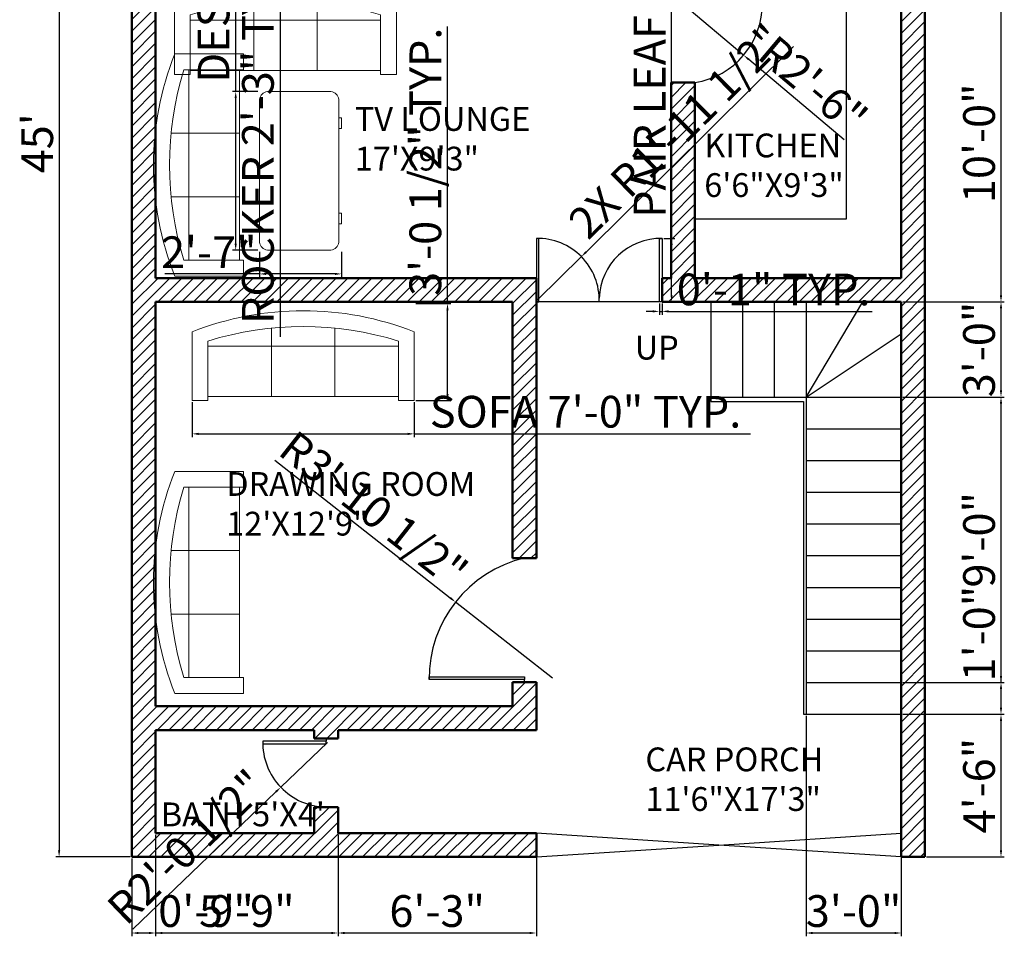
# Model space of a CAD drawing. Units: inches. Extents: x 2308 to 2824, y 1390 to 2024.
# Tile 1 of 2: x 2310 to 2682, y 1390 to 1737. Entities that reach past the tile are written whole.
import ezdxf

# ---------------------------------------------------------------- set-up
doc = ezdxf.new("R2010")
doc.units = ezdxf.units.IN
for name, color, linetype, lineweight in [('A-ANNO-DIMS', 2, 'Continuous', 18), ('A-DOOR', 4, 'Continuous', 25), ('A-FLOR-FIXT', 9, 'Continuous', 25), ('A-FLOR-STRS', 7, 'Continuous', 25), ('A-FURN', 8, 'Continuous', 18), ('A-WALL', 7, 'Continuous', 50)]:
    doc.layers.add(name, color=color, linetype=linetype, lineweight=lineweight)
for name, color, linetype, lineweight, true_color in [('A-ANNO-TEXT', 244, 'Continuous', 25, 0x991b1e), ('A-AREA-IDEN', 244, 'Continuous', 25, 0x991b1e), ('A-WALL-PATT', 177, 'Continuous', 13, 0x293189)]:
    doc.layers.add(name, color=color, linetype=linetype, lineweight=lineweight, true_color=true_color)
doc.styles.get("Standard").update_dxf_attribs({"font": 'arial.ttf'})
doc.dimstyles.new('ISO-25', dxfattribs={"dimtxt": 12, "dimasz": 2.5, "dimexe": 1.25, "dimexo": 0.625, "dimtad": 1, "dimdec": 1, "dimlunit": 3, "dimtxsty": 'Standard', "dimcen": 2.5, "dimadec": 0, "dimazin": 0, "dimtfac": 1, "dimtdec": 1, "dimtmove": 0, "dimatfit": 3, "dimfxl": 1, "dimarcsym": 0})

# ---------------------------------------------------------------- blocks, each defined once
blk = doc.blocks.new('*D2')
at = {"layer": 'A-ANNO-DIMS', "color": 0, "lineweight": -2, "transparency": 16777216}
for p, q in [((2351.84, 1960.47), (2323.71, 1960.47)), ((2324.96, 1957.97), (2324.96, 1422.97)), ((2351.84, 1420.47), (2323.71, 1420.47))]:
    blk.add_line(p, q, dxfattribs=at)
at = {"layer": 'A-ANNO-DIMS', "color": 0, "transparency": 16777216}
for points in [[(2324.54, 1957.97), (2325.37, 1957.97), (2324.96, 1960.47)], [(2324.54, 1422.97), (2325.37, 1422.97), (2324.96, 1420.47)]]:
    blk.add_solid(points, dxfattribs=at)
at = {"layer": 'Defpoints', "color": 0, "transparency": 16777216}
for p in [(2352.46, 1960.47), (2324.96, 1420.47), (2352.46, 1420.47)]:
    blk.add_point(p, dxfattribs=at)
at = {"layer": 'A-ANNO-DIMS', "color": 0, "transparency": 16777216, "insert": (2318.23, 1690.47), "char_height": 12, "attachment_point": 5, "rotation": 90}
blk.add_mtext("45'", dxfattribs=at)
blk = doc.blocks.new('Sofa - Roundback 7 ft.')
for p, q in [((-12.00002, -32.4421), (-12.00003, -6.5971)), ((11.99997, -32.4421), (11.99998, -6.5971)), ((-36.000027, -34), (-36.000027, -11.4696)), ((-35.999844, -13.3819), (35.9998, -13.3819)), ((35.99998, -34), (35.99998, -11.4696)), ((-36.000027, -32.4421), (35.99998, -32.4421))]:
    blk.add_line(p, q)
for points in [[(-36.000027, -34), (-42.000027, -34), (-42.000027, -8)], [(41.99998, -8), (41.99998, -34), (35.99998, -34)]]:
    blk.add_lwpolyline(points)
for centre, radius, start, end in [((0, -114.25), 114.25, 68.43141, 111.5686), ((-0.00001, -127.1968), 121.1968, 72.72033, 107.2797)]:
    blk.add_arc(centre, radius, start, end)
blk = doc.blocks.new('Desk - 30 x 60 in.')
for p, q in [((-26.999995, 0), (26.999995, 0)), ((-29.999995, -27), (-29.999995, -3)), ((29.999995, -3), (29.999995, -27)), ((26.999995, -30), (-26.999995, -30)), ((-20.000005, -30), (-20.000005, -31)), ((-20.000005, -31), (-16.000005, -31)), ((-16.000005, -31), (-16.000005, -30)), ((15.999995, -31), (15.999995, -30)), ((19.999995, -31), (15.999995, -31)), ((19.999995, -30), (19.999995, -31))]:
    blk.add_line(p, q)
for centre, start, end in [((-26.499995, -3.5), 98.1301, 171.8699), ((26.499995, -3.5), 8.130102, 81.8699), ((-26.499995, -26.5), 188.1301, 261.8699), ((26.499995, -26.5), 278.1301, 351.8699)]:
    blk.add_arc(centre, 3.535534, start, end)
blk = doc.blocks.new('DOOR-LEAF-36IN')
for p, q in [((-1, 36), (-2, 36)), ((-2, 36), (-2, 0)), ((-1, 0), (-1, 36)), ((-2, 0), (-1, 0)), ((0, 0), (-1, 0))]:
    blk.add_line(p, q)
blk = doc.blocks.new('DOOR-LEAF-24IN')
for p, q in [((0, 0), (0, -1)), ((0, -1), (-24, -1)), ((-24, -1), (-24, -2)), ((-24, -2), (0, -2)), ((0, -2), (0, -1))]:
    blk.add_line(p, q)
blk = doc.blocks.new('DOOR-PAIR-LEAF-24IN')
for p, q in [((-1, 0), (-1, 24)), ((-1, 24), (0, 24)), ((0, 24), (0, 9)), ((0, 0), (-1, 0))]:
    blk.add_line(p, q)
blk = doc.blocks.new('*D11')
at = {"layer": 'A-ANNO-DIMS', "color": 0, "lineweight": -2, "transparency": 16777216}
for p, q in [((2411.97, 1796.88), (2407.29, 1796.88)), ((2408.54, 1794.38), (2408.54, 1772.38)), ((2411.97, 1769.88), (2407.29, 1769.88)), ((2408.54, 1769.88), (2408.54, 1617.23))]:
    blk.add_line(p, q, dxfattribs=at)
at = {"layer": 'A-ANNO-DIMS', "color": 0, "transparency": 16777216}
for points in [[(2408.13, 1794.38), (2408.96, 1794.38), (2408.54, 1796.88)], [(2408.13, 1772.38), (2408.96, 1772.38), (2408.54, 1769.88)]]:
    blk.add_solid(points, dxfattribs=at)
at = {"layer": 'Defpoints', "color": 0, "transparency": 16777216}
for p in [(2412.59, 1796.88), (2408.54, 1769.88), (2412.59, 1769.88)]:
    blk.add_point(p, dxfattribs=at)
at = {"layer": 'A-ANNO-DIMS', "color": 0, "transparency": 16777216, "insert": (2401.7, 1692.31), "char_height": 12, "attachment_point": 5, "rotation": 90}
blk.add_mtext('ROCKER 2\'-3" TYP.', dxfattribs=at)
blk = doc.blocks.new('*D13')
at = {"layer": 'A-ANNO-DIMS', "color": 0, "lineweight": -2, "transparency": 16777216}
for p, q in [((2375.27, 1592.5), (2375.27, 1579.28)), ((2459.27, 1592.5), (2459.27, 1579.28)), ((2377.77, 1580.53), (2456.77, 1580.53)), ((2459.27, 1580.53), (2586.4, 1580.53))]:
    blk.add_line(p, q, dxfattribs=at)
at = {"layer": 'A-ANNO-DIMS', "color": 0, "transparency": 16777216}
for points in [[(2377.77, 1580.95), (2377.77, 1580.11), (2375.27, 1580.53)], [(2456.77, 1580.95), (2456.77, 1580.11), (2459.27, 1580.53)]]:
    blk.add_solid(points, dxfattribs=at)
at = {"layer": 'Defpoints', "color": 0, "transparency": 16777216}
for p in [(2375.27, 1593.13), (2459.27, 1593.13), (2459.27, 1580.53)]:
    blk.add_point(p, dxfattribs=at)
at = {"layer": 'A-ANNO-DIMS', "color": 0, "transparency": 16777216, "insert": (2524.08, 1587.36), "char_height": 12, "attachment_point": 5}
blk.add_mtext('SOFA 7\'-0" TYP.', dxfattribs=at)
blk = doc.blocks.new('*D14')
at = {"layer": 'A-ANNO-DIMS', "color": 0, "lineweight": -2, "transparency": 16777216}
for p, q in [((2471.87, 1629.8), (2471.87, 1734.65)), ((2459.89, 1629.8), (2473.12, 1629.8)), ((2471.87, 1595.63), (2471.87, 1627.3)), ((2459.89, 1593.13), (2473.12, 1593.13))]:
    blk.add_line(p, q, dxfattribs=at)
at = {"layer": 'A-ANNO-DIMS', "color": 0, "transparency": 16777216}
for points in [[(2471.45, 1627.3), (2472.28, 1627.3), (2471.87, 1629.8)], [(2471.45, 1595.63), (2472.28, 1595.63), (2471.87, 1593.13)]]:
    blk.add_solid(points, dxfattribs=at)
at = {"layer": 'Defpoints', "color": 0, "transparency": 16777216}
for p in [(2459.27, 1629.8), (2471.87, 1629.8), (2459.27, 1593.13)]:
    blk.add_point(p, dxfattribs=at)
at = {"layer": 'A-ANNO-DIMS', "color": 0, "transparency": 16777216, "insert": (2465.03, 1683.47), "char_height": 12, "attachment_point": 5, "rotation": 90}
blk.add_mtext('3\'-0 1/2" TYP.', dxfattribs=at)
blk = doc.blocks.new('*D17')
at = {"layer": 'A-ANNO-DIMS', "color": 0, "lineweight": -2, "transparency": 16777216}
for p, q in [((2391.75, 1710.04), (2391.75, 1795.4)), ((2400.13, 1710.04), (2390.5, 1710.04)), ((2391.75, 1652.54), (2391.75, 1707.54)), ((2400.13, 1650.04), (2390.5, 1650.04))]:
    blk.add_line(p, q, dxfattribs=at)
at = {"layer": 'A-ANNO-DIMS', "color": 0, "transparency": 16777216}
for points in [[(2391.34, 1707.54), (2392.17, 1707.54), (2391.75, 1710.04)], [(2391.34, 1652.54), (2392.17, 1652.54), (2391.75, 1650.04)]]:
    blk.add_solid(points, dxfattribs=at)
at = {"layer": 'Defpoints', "color": 0, "transparency": 16777216}
for p in [(2391.75, 1710.04), (2400.75, 1710.04), (2400.75, 1650.04)]:
    blk.add_point(p, dxfattribs=at)
at = {"layer": 'A-ANNO-DIMS', "color": 0, "transparency": 16777216, "insert": (2384.92, 1753.97), "char_height": 12, "attachment_point": 5, "rotation": 90}
blk.add_mtext('DESK 5\'-0"', dxfattribs=at)
blk = doc.blocks.new('*D18')
at = {"layer": 'A-ANNO-DIMS', "color": 0, "lineweight": -2, "transparency": 16777216}
for p, q in [((2400.75, 1649.42), (2400.75, 1639.79)), ((2431.75, 1649.42), (2431.75, 1639.79)), ((2400.75, 1641.04), (2364.9, 1641.04)), ((2429.25, 1641.04), (2403.25, 1641.04))]:
    blk.add_line(p, q, dxfattribs=at)
at = {"layer": 'A-ANNO-DIMS', "color": 0, "transparency": 16777216}
for points in [[(2403.25, 1641.46), (2403.25, 1640.63), (2400.75, 1641.04)], [(2429.25, 1641.46), (2429.25, 1640.63), (2431.75, 1641.04)]]:
    blk.add_solid(points, dxfattribs=at)
at = {"layer": 'Defpoints', "color": 0, "transparency": 16777216}
for p in [(2400.75, 1650.04), (2431.75, 1650.04), (2400.75, 1641.04)]:
    blk.add_point(p, dxfattribs=at)
at = {"layer": 'A-ANNO-DIMS', "color": 0, "transparency": 16777216, "insert": (2381.58, 1647.69), "char_height": 12, "attachment_point": 5}
blk.add_mtext('2\'-7"', dxfattribs=at)
blk = doc.blocks.new('*D23')
at = {"layer": 'A-ANNO-DIMS', "color": 0, "lineweight": -2, "transparency": 16777216}
for p, q in [((2556.62, 1654.47), (2556.62, 1821.13)), ((2553.65, 1654.47), (2557.87, 1654.47)), ((2556.62, 1632.97), (2556.62, 1651.97)), ((2553.65, 1630.47), (2557.87, 1630.47))]:
    blk.add_line(p, q, dxfattribs=at)
at = {"layer": 'A-ANNO-DIMS', "color": 0, "transparency": 16777216}
for points in [[(2556.21, 1651.97), (2557.04, 1651.97), (2556.62, 1654.47)], [(2556.21, 1632.97), (2557.04, 1632.97), (2556.62, 1630.47)]]:
    blk.add_solid(points, dxfattribs=at)
at = {"layer": 'Defpoints', "color": 0, "transparency": 16777216}
for p in [(2553.02, 1654.47), (2556.62, 1654.47), (2553.02, 1630.47)]:
    blk.add_point(p, dxfattribs=at)
at = {"layer": 'A-ANNO-DIMS', "color": 0, "transparency": 16777216, "insert": (2549.87, 1739.05), "char_height": 12, "attachment_point": 5, "rotation": 90}
blk.add_mtext('PAIR LEAF 2\'-0" TYP.', dxfattribs=at)
blk = doc.blocks.new('*D24')
at = {"layer": 'A-ANNO-DIMS', "color": 0, "lineweight": -2, "transparency": 16777216}
for p, q in [((2552.02, 1629.84), (2552.02, 1625.62)), ((2553.02, 1629.84), (2553.02, 1625.62)), ((2549.52, 1626.87), (2547.02, 1626.87)), ((2552.02, 1626.87), (2553.02, 1626.87)), ((2555.52, 1626.87), (2632.42, 1626.87))]:
    blk.add_line(p, q, dxfattribs=at)
at = {"layer": 'A-ANNO-DIMS', "color": 0, "transparency": 16777216}
for points in [[(2549.52, 1627.28), (2549.52, 1626.45), (2552.02, 1626.87)], [(2555.52, 1627.28), (2555.52, 1626.45), (2553.02, 1626.87)]]:
    blk.add_solid(points, dxfattribs=at)
at = {"layer": 'Defpoints', "color": 0, "transparency": 16777216}
for p in [(2552.02, 1630.47), (2553.02, 1630.47), (2553.02, 1626.87)]:
    blk.add_point(p, dxfattribs=at)
at = {"layer": 'A-ANNO-DIMS', "color": 0, "transparency": 16777216, "insert": (2595.22, 1633.62), "char_height": 12, "attachment_point": 5}
blk.add_mtext('0\'-1" TYP.', dxfattribs=at)
blk = doc.blocks.new('*D25')
at = {"layer": 'A-ANNO-DIMS', "color": 0, "lineweight": -2, "transparency": 16777216}
for p, q in [((2361.46, 1428.84), (2361.46, 1390.47)), ((2352.46, 1419.84), (2352.46, 1390.47)), ((2354.96, 1391.72), (2358.96, 1391.72)), ((2361.46, 1391.72), (2397.11, 1391.72))]:
    blk.add_line(p, q, dxfattribs=at)
at = {"layer": 'A-ANNO-DIMS', "color": 0, "transparency": 16777216}
for points in [[(2354.96, 1392.13), (2354.96, 1391.3), (2352.46, 1391.72)], [(2358.96, 1392.13), (2358.96, 1391.3), (2361.46, 1391.72)]]:
    blk.add_solid(points, dxfattribs=at)
at = {"layer": 'Defpoints', "color": 0, "transparency": 16777216}
for p in [(2361.46, 1429.47), (2352.46, 1420.47), (2361.46, 1391.72)]:
    blk.add_point(p, dxfattribs=at)
at = {"layer": 'A-ANNO-DIMS', "color": 0, "transparency": 16777216, "insert": (2380.53, 1398.47), "char_height": 12, "attachment_point": 5}
blk.add_mtext('0\'-9"', dxfattribs=at)
blk = doc.blocks.new('*D26')
at = {"layer": 'A-ANNO-DIMS', "color": 0, "lineweight": -2, "transparency": 16777216}
for p, q in [((2361.46, 1428.84), (2361.46, 1390.47)), ((2430.46, 1428.84), (2430.46, 1390.47)), ((2363.96, 1391.72), (2427.96, 1391.72))]:
    blk.add_line(p, q, dxfattribs=at)
at = {"layer": 'A-ANNO-DIMS', "color": 0, "transparency": 16777216}
for points in [[(2363.96, 1392.13), (2363.96, 1391.3), (2361.46, 1391.72)], [(2427.96, 1392.13), (2427.96, 1391.3), (2430.46, 1391.72)]]:
    blk.add_solid(points, dxfattribs=at)
at = {"layer": 'Defpoints', "color": 0, "transparency": 16777216}
for p in [(2361.46, 1429.47), (2430.46, 1429.47), (2430.46, 1391.72)]:
    blk.add_point(p, dxfattribs=at)
at = {"layer": 'A-ANNO-DIMS', "color": 0, "transparency": 16777216, "insert": (2395.96, 1398.47), "char_height": 12, "attachment_point": 5}
blk.add_mtext('5\'-9"', dxfattribs=at)
blk = doc.blocks.new('*D27')
at = {"layer": 'A-ANNO-DIMS', "color": 0, "lineweight": -2, "transparency": 16777216}
for p, q in [((2430.46, 1428.84), (2430.46, 1390.47)), ((2505.46, 1428.84), (2505.46, 1390.47)), ((2432.96, 1391.72), (2502.96, 1391.72))]:
    blk.add_line(p, q, dxfattribs=at)
at = {"layer": 'A-ANNO-DIMS', "color": 0, "transparency": 16777216}
for points in [[(2432.96, 1392.13), (2432.96, 1391.3), (2430.46, 1391.72)], [(2502.96, 1392.13), (2502.96, 1391.3), (2505.46, 1391.72)]]:
    blk.add_solid(points, dxfattribs=at)
at = {"layer": 'Defpoints', "color": 0, "transparency": 16777216}
for p in [(2430.46, 1429.47), (2505.46, 1429.47), (2505.46, 1391.72)]:
    blk.add_point(p, dxfattribs=at)
at = {"layer": 'A-ANNO-DIMS', "color": 0, "transparency": 16777216, "insert": (2467.96, 1398.47), "char_height": 12, "attachment_point": 5}
blk.add_mtext('6\'-3"', dxfattribs=at)
blk = doc.blocks.new('*D28')
at = {"layer": 'A-ANNO-DIMS', "color": 0, "lineweight": -2, "transparency": 16777216}
for p, q in [((2607.46, 1473.84), (2607.46, 1390.47)), ((2643.46, 1473.84), (2643.46, 1390.47)), ((2609.96, 1391.72), (2640.96, 1391.72))]:
    blk.add_line(p, q, dxfattribs=at)
at = {"layer": 'A-ANNO-DIMS', "color": 0, "transparency": 16777216}
for points in [[(2609.96, 1392.13), (2609.96, 1391.3), (2607.46, 1391.72)], [(2640.96, 1392.13), (2640.96, 1391.3), (2643.46, 1391.72)]]:
    blk.add_solid(points, dxfattribs=at)
at = {"layer": 'Defpoints', "color": 0, "transparency": 16777216}
for p in [(2607.46, 1474.47), (2643.46, 1474.47), (2643.46, 1391.72)]:
    blk.add_point(p, dxfattribs=at)
at = {"layer": 'A-ANNO-DIMS', "color": 0, "transparency": 16777216, "insert": (2625.46, 1398.47), "char_height": 12, "attachment_point": 5}
blk.add_mtext('3\'-0"', dxfattribs=at)
blk = doc.blocks.new('*D29')
at = {"layer": 'A-ANNO-DIMS', "color": 0, "lineweight": -2, "transparency": 16777216}
for p, q in [((2644.09, 1474.47), (2682.46, 1474.47)), ((2681.21, 1422.97), (2681.21, 1471.97)), ((2653.09, 1420.47), (2682.46, 1420.47))]:
    blk.add_line(p, q, dxfattribs=at)
at = {"layer": 'A-ANNO-DIMS', "color": 0, "transparency": 16777216}
for points in [[(2680.79, 1471.97), (2681.63, 1471.97), (2681.21, 1474.47)], [(2680.79, 1422.97), (2681.63, 1422.97), (2681.21, 1420.47)]]:
    blk.add_solid(points, dxfattribs=at)
at = {"layer": 'Defpoints', "color": 0, "transparency": 16777216}
for p in [(2643.46, 1474.47), (2681.21, 1474.47), (2652.46, 1420.47)]:
    blk.add_point(p, dxfattribs=at)
at = {"layer": 'A-ANNO-DIMS', "color": 0, "transparency": 16777216, "insert": (2674.46, 1447.47), "char_height": 12, "attachment_point": 5, "rotation": 90}
blk.add_mtext('4\'-6"', dxfattribs=at)
blk = doc.blocks.new('*D30')
at = {"layer": 'A-ANNO-DIMS', "color": 0, "lineweight": -2, "transparency": 16777216}
for p, q in [((2681.21, 1486.47), (2681.21, 1520.99)), ((2644.09, 1486.47), (2682.46, 1486.47)), ((2681.21, 1476.97), (2681.21, 1483.97)), ((2644.09, 1474.47), (2682.46, 1474.47))]:
    blk.add_line(p, q, dxfattribs=at)
at = {"layer": 'A-ANNO-DIMS', "color": 0, "transparency": 16777216}
for points in [[(2680.79, 1483.97), (2681.63, 1483.97), (2681.21, 1486.47)], [(2680.79, 1476.97), (2681.63, 1476.97), (2681.21, 1474.47)]]:
    blk.add_solid(points, dxfattribs=at)
at = {"layer": 'Defpoints', "color": 0, "transparency": 16777216}
for p in [(2643.46, 1486.47), (2681.21, 1486.47), (2643.46, 1474.47)]:
    blk.add_point(p, dxfattribs=at)
at = {"layer": 'A-ANNO-DIMS', "color": 0, "transparency": 16777216, "insert": (2674.46, 1504.98), "char_height": 12, "attachment_point": 5, "rotation": 90}
blk.add_mtext('1\'-0"', dxfattribs=at)
blk = doc.blocks.new('*D31')
at = {"layer": 'A-ANNO-DIMS', "color": 0, "lineweight": -2, "transparency": 16777216}
for p, q in [((2644.09, 1594.47), (2682.46, 1594.47)), ((2681.21, 1488.97), (2681.21, 1591.97)), ((2644.09, 1486.47), (2682.46, 1486.47))]:
    blk.add_line(p, q, dxfattribs=at)
at = {"layer": 'A-ANNO-DIMS', "color": 0, "transparency": 16777216}
for points in [[(2680.79, 1591.97), (2681.63, 1591.97), (2681.21, 1594.47)], [(2680.79, 1488.97), (2681.63, 1488.97), (2681.21, 1486.47)]]:
    blk.add_solid(points, dxfattribs=at)
at = {"layer": 'Defpoints', "color": 0, "transparency": 16777216}
for p in [(2643.46, 1594.47), (2681.21, 1594.47), (2643.46, 1486.47)]:
    blk.add_point(p, dxfattribs=at)
at = {"layer": 'A-ANNO-DIMS', "color": 0, "transparency": 16777216, "insert": (2674.46, 1540.47), "char_height": 12, "attachment_point": 5, "rotation": 90}
blk.add_mtext('9\'-0"', dxfattribs=at)
blk = doc.blocks.new('*D32')
at = {"layer": 'A-ANNO-DIMS', "color": 0, "lineweight": -2, "transparency": 16777216}
for p, q in [((2644.09, 1630.47), (2682.46, 1630.47)), ((2681.21, 1596.97), (2681.21, 1627.97)), ((2644.09, 1594.47), (2682.46, 1594.47))]:
    blk.add_line(p, q, dxfattribs=at)
at = {"layer": 'A-ANNO-DIMS', "color": 0, "transparency": 16777216}
for points in [[(2680.79, 1627.97), (2681.63, 1627.97), (2681.21, 1630.47)], [(2680.79, 1596.97), (2681.63, 1596.97), (2681.21, 1594.47)]]:
    blk.add_solid(points, dxfattribs=at)
at = {"layer": 'Defpoints', "color": 0, "transparency": 16777216}
for p in [(2643.46, 1630.47), (2681.21, 1630.47), (2643.46, 1594.47)]:
    blk.add_point(p, dxfattribs=at)
at = {"layer": 'A-ANNO-DIMS', "color": 0, "transparency": 16777216, "insert": (2674.45, 1612.47), "char_height": 12, "attachment_point": 5, "rotation": 90}
blk.add_mtext('3\'-0"', dxfattribs=at)
blk = doc.blocks.new('*D33')
at = {"layer": 'A-ANNO-DIMS', "color": 0, "lineweight": -2, "transparency": 16777216}
for p, q in [((2644.09, 1750.47), (2682.46, 1750.47)), ((2681.21, 1632.97), (2681.21, 1747.97)), ((2644.09, 1630.47), (2682.46, 1630.47))]:
    blk.add_line(p, q, dxfattribs=at)
at = {"layer": 'A-ANNO-DIMS', "color": 0, "transparency": 16777216}
for points in [[(2680.79, 1747.97), (2681.63, 1747.97), (2681.21, 1750.47)], [(2680.79, 1632.97), (2681.63, 1632.97), (2681.21, 1630.47)]]:
    blk.add_solid(points, dxfattribs=at)
at = {"layer": 'Defpoints', "color": 0, "transparency": 16777216}
for p in [(2643.46, 1750.47), (2681.21, 1750.47), (2643.46, 1630.47)]:
    blk.add_point(p, dxfattribs=at)
at = {"layer": 'A-ANNO-DIMS', "color": 0, "transparency": 16777216, "insert": (2674.46, 1690.47), "char_height": 12, "attachment_point": 5, "rotation": 90}
blk.add_mtext('10\'-0"', dxfattribs=at)
blk = doc.blocks.new('*D36')
at = {"layer": 'A-ANNO-DIMS', "color": 0, "lineweight": -2, "transparency": 16777216}
for p, q in [((2406.51, 1570.57), (2472.93, 1518.46)), ((2511.57, 1488.15), (2474.9, 1516.92))]:
    blk.add_line(p, q, dxfattribs=at)
at = {"layer": 'A-ANNO-DIMS', "color": 0, "transparency": 16777216}
blk.add_solid([(2473.19, 1518.79), (2472.67, 1518.13), (2474.9, 1516.92)], dxfattribs=at)
at = {"layer": 'Defpoints', "color": 0, "transparency": 16777216}
for p in [(2474.9, 1516.92), (2511.57, 1488.15)]:
    blk.add_point(p, dxfattribs=at)
at = {"layer": 'A-ANNO-DIMS', "color": 0, "transparency": 16777216, "insert": (2442.96, 1550.66), "char_height": 12, "attachment_point": 5, "rotation": 321.8845}
blk.add_mtext('R3\'-10 1/2"', dxfattribs=at)
blk = doc.blocks.new('*D39')
at = {"layer": 'A-ANNO-DIMS', "color": 0, "lineweight": -2, "transparency": 16777216}
for p, q in [((2560.86, 1743.18), (2583.88, 1723.78)), ((2621.83, 1691.79), (2585.79, 1722.17))]:
    blk.add_line(p, q, dxfattribs=at)
at = {"layer": 'A-ANNO-DIMS', "color": 0, "transparency": 16777216}
blk.add_solid([(2586.06, 1722.48), (2585.52, 1721.85), (2583.88, 1723.78)], dxfattribs=at)
at = {"layer": 'Defpoints', "color": 0, "transparency": 16777216}
for p in [(2560.86, 1743.18), (2583.88, 1723.78)]:
    blk.add_point(p, dxfattribs=at)
at = {"layer": 'A-ANNO-DIMS', "color": 0, "transparency": 16777216, "insert": (2609.12, 1711.33), "char_height": 12, "attachment_point": 5, "rotation": 319.8697}
blk.add_mtext('R2\'-6"', dxfattribs=at)
blk = doc.blocks.new('*D41')
at = {"layer": 'A-ANNO-DIMS', "color": 0, "lineweight": -2, "transparency": 16777216}
for p, q in [((2426.45, 1463.83), (2408.78, 1446.86)), ((2352.82, 1393.11), (2406.98, 1445.13))]:
    blk.add_line(p, q, dxfattribs=at)
at = {"layer": 'A-ANNO-DIMS', "color": 0, "transparency": 16777216}
blk.add_solid([(2406.69, 1445.43), (2407.27, 1444.83), (2408.78, 1446.86)], dxfattribs=at)
at = {"layer": 'Defpoints', "color": 0, "transparency": 16777216}
for p in [(2426.45, 1463.83), (2408.78, 1446.86)]:
    blk.add_point(p, dxfattribs=at)
at = {"layer": 'A-ANNO-DIMS', "color": 0, "transparency": 16777216, "insert": (2374.27, 1423.18), "char_height": 12, "attachment_point": 5, "rotation": 43.8411}
blk.add_mtext('R2\'-0 1/2"', dxfattribs=at)
blk = doc.blocks.new('*D42')
at = {"layer": 'A-ANNO-DIMS', "color": 0, "lineweight": -2, "transparency": 16777216}
for p, q in [((2602.71, 1727.05), (2524.28, 1649.33)), ((2505.96, 1631.18), (2522.51, 1647.57))]:
    blk.add_line(p, q, dxfattribs=at)
at = {"layer": 'A-ANNO-DIMS', "color": 0, "transparency": 16777216}
blk.add_solid([(2523.99, 1649.63), (2524.57, 1649.04), (2522.51, 1647.57)], dxfattribs=at)
at = {"layer": 'Defpoints', "color": 0, "transparency": 16777216}
for p in [(2522.51, 1647.57), (2505.96, 1631.18)]:
    blk.add_point(p, dxfattribs=at)
at = {"layer": 'A-ANNO-DIMS', "color": 0, "transparency": 16777216, "insert": (2559.57, 1693.92), "char_height": 12, "attachment_point": 5, "rotation": 44.7381}
blk.add_mtext('2X R1\'-11 1/2"', dxfattribs=at)

msp = doc.modelspace()

# ---------------------------------------------------------------- hatches: boundary and pattern name
at = {"layer": 'A-WALL-PATT'}
h = msp.add_hatch(dxfattribs=at)
h.set_pattern_fill('ANSI31', color=256)
h.paths.add_polyline_path([(2361.46, 1750.47), (2459.65, 1750.47), (2459.65, 1759.47), (2361.46, 1759.47), (2361.46, 1903.47), (2454.46, 1903.47), (2454.46, 1912.24), (2361.46, 1912.47), (2361.46, 1951.47), (2445.46, 1951.47), (2445.46, 1945.01), (2454.46, 1945.01), (2454.46, 1951.47), (2643.46, 1951.47), (2643.46, 1912.47), (2635.92, 1912.47), (2635.92, 1903.47), (2643.46, 1903.47), (2643.46, 1759.47), (2554.14, 1759.47), (2554.14, 1750.47), (2556.46, 1750.47), (2556.46, 1744.68), (2565.46, 1744.68), (2565.46, 1750.47), (2643.46, 1750.47), (2643.46, 1639.47), (2565.46, 1639.47), (2565.46, 1713.43), (2556.46, 1713.43), (2556.46, 1639.47), (2553.02, 1639.47), (2553.02, 1630.47), (2643.46, 1630.47), (2643.46, 1429.47), (2643.46, 1420.47), (2652.46, 1420.47), (2652.46, 1960.47), (2352.46, 1960.47), (2352.46, 1420.47), (2505.46, 1420.47), (2505.46, 1429.47), (2430.46, 1429.47), (2430.46, 1439.34), (2421.46, 1439.34), (2421.46, 1429.47), (2361.46, 1429.47), (2361.46, 1468.47), (2421.46, 1468.47), (2421.46, 1465.33), (2430.46, 1465.33), (2430.46, 1468.47), (2505.46, 1468.47), (2505.46, 1477.47), (2505.46, 1486.65), (2496.46, 1486.65), (2496.46, 1477.47), (2361.46, 1477.47), (2361.46, 1630.47), (2496.46, 1630.47), (2496.46, 1533.54), (2505.46, 1533.54), (2505.46, 1630.47), (2505.46, 1639.47), (2503.24, 1639.47), (2361.46, 1639.47)])
h.paths.add_polyline_path([(2511.46, 1903.47), (2502.46, 1903.47), (2502.46, 1759.47), (2497.04, 1759.47), (2497.04, 1750.47), (2514.9, 1750.47), (2514.9, 1759.47), (2511.46, 1759.47)], flags=17)
h.paths.add_polyline_path([(2608.34, 1912.47), (2559.46, 1912.47), (2559.46, 1951.47), (2550.46, 1951.47), (2550.46, 1912.47), (2497.43, 1912.47), (2497.43, 1903.47), (2608.44, 1903.47), (2608.44, 1907.97, -0.041548)], flags=17)
h.paths.add_polyline_path([(2360.24, 1427.17), (2428.94, 1427.17), (2428.94, 1445.72), (2360.24, 1445.72)], flags=24)

# ---------------------------------------------------------------- linework, layer by layer
at = {"layer": 'A-DOOR'}
for p, q in [((2553.02, 1630.47), (2505.46, 1630.47)), ((2574.46, 1424.97), (2505.46, 1429.47)), ((2574.46, 1424.97), (2643.46, 1429.47)), ((2505.46, 1420.47), (2574.46, 1424.97)), ((2643.46, 1420.47), (2574.46, 1424.97))]:
    msp.add_line(p, q, dxfattribs=at)
for centre, radius, start, end in [((2560.86, 1743.18), 30.1, 278.7856, 0.9517), ((2505.96, 1631.18), 23.29, 358.2443, 91.2301), ((2552.52, 1631.18), 23.29, 88.7699, 178.2443), ((2511.57, 1488.15), 46.61, 103.1548, 180.6146), ((2426.45, 1463.83), 24.5, 178.8305, 268.8502)]:
    msp.add_arc(centre, radius, start, end, dxfattribs=at)
at = {"layer": 'A-FLOR-FIXT'}
for p, q in [((2622.77, 1661.84), (2622.77, 1750.47)), ((2565.46, 1661.84), (2622.77, 1661.84))]:
    msp.add_line(p, q, dxfattribs=at)
at = {"layer": 'A-FLOR-STRS'}
for p, q in [((2571.46, 1630.47), (2571.46, 1594.47)), ((2583.46, 1630.47), (2583.46, 1594.47)), ((2595.46, 1630.47), (2595.46, 1594.47)), ((2607.46, 1630.47), (2607.46, 1474.47)), ((2607.46, 1594.47), (2628.91, 1630.47)), ((2607.46, 1594.47), (2643.46, 1618.32)), ((2571.46, 1594.47), (2643.46, 1594.47)), ((2571.46, 1594.47), (2571.46, 1592.83)), ((2571.46, 1592.83), (2606.49, 1592.83)), ((2606.49, 1592.83), (2606.49, 1474.47)), ((2607.46, 1582.47), (2643.46, 1582.47)), ((2607.46, 1570.47), (2643.46, 1570.47)), ((2607.46, 1558.47), (2643.46, 1558.47)), ((2607.46, 1546.47), (2643.46, 1546.47)), ((2607.46, 1534.47), (2643.46, 1534.47)), ((2607.46, 1522.47), (2643.46, 1522.47)), ((2607.46, 1510.47), (2643.46, 1510.47)), ((2607.46, 1498.47), (2643.46, 1498.47)), ((2607.46, 1486.47), (2643.46, 1486.47)), ((2606.49, 1474.47), (2607.46, 1474.47)), ((2607.46, 1474.47), (2643.46, 1474.47))]:
    msp.add_line(p, q, dxfattribs=at)
at = {"layer": 'A-WALL'}
for p, q in [((2352.46, 1420.47), (2352.46, 1960.47)), ((2652.46, 1960.47), (2652.46, 1420.47)), ((2361.46, 1639.47), (2361.46, 1750.47)), ((2643.46, 1750.47), (2643.46, 1639.47)), ((2565.46, 1713.43), (2556.46, 1713.43)), ((2556.46, 1713.43), (2556.46, 1639.47)), ((2565.46, 1713.43), (2565.46, 1639.47)), ((2361.46, 1639.47), (2503.24, 1639.47)), ((2505.46, 1639.47), (2503.24, 1639.47)), ((2505.46, 1630.47), (2505.46, 1639.47)), ((2553.02, 1639.47), (2553.02, 1630.47)), ((2553.02, 1639.47), (2556.46, 1639.47)), ((2565.46, 1639.47), (2643.46, 1639.47)), ((2361.46, 1630.47), (2496.46, 1630.47)), ((2361.46, 1477.47), (2361.46, 1630.47)), ((2496.46, 1533.54), (2496.46, 1630.47)), ((2505.46, 1533.54), (2505.46, 1630.47)), ((2553.02, 1630.47), (2643.46, 1630.47)), ((2643.46, 1630.47), (2643.46, 1429.47)), ((2505.46, 1533.54), (2496.46, 1533.54)), ((2496.46, 1477.47), (2496.46, 1486.65)), ((2505.46, 1486.65), (2496.46, 1486.65)), ((2505.46, 1477.47), (2505.46, 1486.65)), ((2361.46, 1477.47), (2496.46, 1477.47)), ((2505.46, 1477.47), (2505.46, 1468.47)), ((2361.46, 1429.47), (2361.46, 1468.47)), ((2361.46, 1468.47), (2421.46, 1468.47)), ((2421.46, 1465.33), (2421.46, 1468.47)), ((2430.46, 1465.33), (2430.46, 1468.47)), ((2430.46, 1468.47), (2505.46, 1468.47)), ((2430.46, 1465.33), (2421.46, 1465.33)), ((2421.46, 1429.47), (2421.46, 1439.34)), ((2430.46, 1439.34), (2421.46, 1439.34)), ((2430.46, 1429.47), (2430.46, 1439.34)), ((2421.46, 1429.47), (2361.46, 1429.47)), ((2505.46, 1429.47), (2430.46, 1429.47)), ((2505.46, 1429.47), (2505.46, 1420.47)), ((2643.46, 1429.47), (2643.46, 1420.47)), ((2505.46, 1420.47), (2352.46, 1420.47)), ((2652.46, 1420.47), (2643.46, 1420.47))]:
    msp.add_line(p, q, dxfattribs=at)

# ---------------------------------------------------------------- block references
at = {"layer": 'A-DOOR', "extrusion": (0, 0, -1), "zscale": -1}
msp.add_blockref('DOOR-PAIR-LEAF-24IN', (-2505.46, 1630.47), dxfattribs=at)
at = {"layer": 'A-DOOR'}
for name, p in [('DOOR-PAIR-LEAF-24IN', (2553.02, 1630.47)), ('DOOR-LEAF-24IN', (2425.96, 1465.33))]:
    msp.add_blockref(name, p, dxfattribs=at)
at = {"layer": 'A-DOOR', "extrusion": (0, 0, -1), "zscale": -1, "rotation": 269.9999999999981}
msp.add_blockref('DOOR-LEAF-36IN', (-2500.96, 1486.65), dxfattribs=at)
at = {"layer": 'A-FURN'}
for p in [(2410.55, 1750.47), (2417.27, 1627.13)]:
    msp.add_blockref('Sofa - Roundback 7 ft.', p, dxfattribs=at)
at = {"layer": 'A-FURN', "rotation": 90}
for name, p in [('Sofa - Roundback 7 ft.', (2360.69, 1682.25)), ('Desk - 30 x 60 in.', (2400.75, 1680.04)), ('Sofa - Roundback 7 ft.', (2360.69, 1524.36))]:
    msp.add_blockref(name, p, dxfattribs=at)

# ---------------------------------------------------------------- texts
at = {"layer": 'A-ANNO-TEXT', "insert": (2542.7, 1617.64), "char_height": 9, "attachment_point": 1}
msp.add_mtext_dynamic_manual_height_columns('UP', width=23.1939, gutter_width=12.5, heights=[0], dxfattribs=at)
at = {"layer": 'A-AREA-IDEN', "char_height": 9, "attachment_point": 1}
for s, width, insert in [('TV LOUNGE\\P17\'X9\'3"', 126.5372, (2436.82, 1704.16)), ('KITCHEN\\P6\'6"X9\'3"', 64.432, (2568.98, 1694.14)), ('DRAWING ROOM\\P12\'X12\'9"', 123.9108, (2388.18, 1566.07)), ('CAR PORCH\\P11\'6"X17\'3"', 77.3787, (2546.71, 1461.89)), ("BATH 5'X4'", 64.432, (2363.42, 1441.09))]:
    msp.add_mtext_dynamic_manual_height_columns(s, width=width, gutter_width=12.5, heights=[0], dxfattribs=dict(at, insert=insert))

# ---------------------------------------------------------------- dimensions: what is measured, and where the dimension line sits
at = {"layer": 'A-ANNO-DIMS'}
for base, p1, p2, angle, override, picture, middle in [((2324.96, 1420.47), (2352.46, 1960.47), (2352.46, 1420.47), 90, {"dimclrd": 0, "dimclre": 0, "dimclrt": 0}, '*D2', (2318.23, 1690.47)), ((2681.21, 1750.47), (2643.46, 1630.47), (2643.46, 1750.47), 90, {"dimdec": 1, "dimlfac": 1, "dimrnd": 0, "dimzin": 1, "dimdsep": 46, "dimlunit": 4, "dimfrac": 2}, '*D33', (2674.46, 1690.47)), ((2400.75, 1641.04), (2431.75, 1650.04), (2400.75, 1650.04), 180, {"dimdec": 1, "dimlfac": 1, "dimrnd": 0, "dimzin": 1, "dimdsep": 46, "dimlunit": 4, "dimfrac": 2}, '*D18', (2381.58, 1647.69)), ((2681.21, 1630.47), (2643.46, 1594.47), (2643.46, 1630.47), 90, {"dimdec": 1, "dimlfac": 1, "dimrnd": 0, "dimzin": 1, "dimdsep": 46, "dimlunit": 4, "dimfrac": 2}, '*D32', (2674.45, 1612.47)), ((2681.21, 1594.47), (2643.46, 1486.47), (2643.46, 1594.47), 90, {"dimdec": 1, "dimlfac": 1, "dimrnd": 0, "dimzin": 1, "dimdsep": 46, "dimlunit": 4, "dimfrac": 2}, '*D31', (2674.46, 1540.47)), ((2681.21, 1486.47), (2643.46, 1474.47), (2643.46, 1486.47), 90, {"dimdec": 1, "dimlfac": 1, "dimrnd": 0, "dimzin": 1, "dimdsep": 46, "dimlunit": 4, "dimfrac": 2}, '*D30', (2674.46, 1504.98)), ((2681.21, 1474.47), (2652.46, 1420.47), (2643.46, 1474.47), 90, {"dimdec": 1, "dimlfac": 1, "dimrnd": 0, "dimzin": 1, "dimdsep": 46, "dimlunit": 4, "dimfrac": 2}, '*D29', (2674.46, 1447.47))]:
    dim = msp.add_linear_dim(base=base, p1=p1, p2=p2, angle=angle, dimstyle='ISO-25', override=override, dxfattribs=at)
    dim.commit()
    dim.dimension.update_dxf_attribs({"geometry": picture, "text_midpoint": middle})
for base, p1, p2, angle, text, picture, middle in [((2556.62, 1654.47), (2553.02, 1630.47), (2553.02, 1654.47), 90, 'PAIR LEAF <> TYP.', '*D23', (2549.87, 1739.05)), ((2391.75, 1710.04), (2400.75, 1650.04), (2400.75, 1710.04), 90, 'DESK <>', '*D17', (2384.92, 1753.97)), ((2408.54, 1769.88), (2412.59, 1796.88), (2412.59, 1769.88), 270, 'ROCKER <> TYP.', '*D11', (2401.7, 1692.31)), ((2471.87, 1629.8), (2459.27, 1593.13), (2459.27, 1629.8), 90, '<> TYP.', '*D14', (2465.03, 1683.47))]:
    dim = msp.add_linear_dim(base=base, p1=p1, p2=p2, angle=angle, text=text, dimstyle='ISO-25', override={"dimdec": 1, "dimlfac": 1, "dimrnd": 0, "dimzin": 1, "dimdsep": 46, "dimlunit": 4, "dimfrac": 2}, dxfattribs=at)
    dim.commit()
    dim.dimension.update_dxf_attribs({"geometry": picture, "text_midpoint": middle})
for center, mpoint, picture, middle in [((2560.86, 1743.18), (2583.88, 1723.78), '*D39', (2609.12, 1711.33)), ((2511.57, 1488.15), (2474.9, 1516.92), '*D36', (2442.96, 1550.66)), ((2426.45, 1463.83), (2408.78, 1446.86), '*D41', (2374.27, 1423.18))]:
    dim = msp.add_radius_dim(center=center, mpoint=mpoint, dimstyle='ISO-25', override={"dimdec": 1, "dimlfac": 1, "dimrnd": 0, "dimzin": 1, "dimdsep": 46, "dimlunit": 4, "dimfrac": 2}, dxfattribs=at)
    dim.commit()
    dim.dimension.update_dxf_attribs({"geometry": picture, "text_midpoint": middle})
dim = msp.add_radius_dim(center=(2505.96, 1631.18), mpoint=(2522.51, 1647.57), text='2X <>', dimstyle='ISO-25', override={"dimdec": 1, "dimlfac": 1, "dimrnd": 0, "dimzin": 1, "dimdsep": 46, "dimlunit": 4, "dimfrac": 2}, dxfattribs=at)
dim.commit()
dim.dimension.update_dxf_attribs({"geometry": '*D42', "text_midpoint": (2559.57, 1693.92)})
for base, p1, p2, text, picture, middle in [((2553.02, 1626.87), (2552.02, 1630.47), (2553.02, 1630.47), '<> TYP.', '*D24', (2595.22, 1633.62)), ((2459.27, 1580.53), (2375.27, 1593.13), (2459.27, 1593.13), 'SOFA <> TYP.', '*D13', (2524.08, 1587.36))]:
    dim = msp.add_linear_dim(base=base, p1=p1, p2=p2, text=text, dimstyle='ISO-25', override={"dimdec": 1, "dimlfac": 1, "dimrnd": 0, "dimzin": 1, "dimdsep": 46, "dimlunit": 4, "dimfrac": 2}, dxfattribs=at)
    dim.commit()
    dim.dimension.update_dxf_attribs({"geometry": picture, "text_midpoint": middle})
for base, p1, p2, picture, middle in [((2643.46, 1391.72), (2607.46, 1474.47), (2643.46, 1474.47), '*D28', (2625.46, 1398.47)), ((2361.46, 1391.72), (2352.46, 1420.47), (2361.46, 1429.47), '*D25', (2380.53, 1398.47)), ((2430.46, 1391.72), (2361.46, 1429.47), (2430.46, 1429.47), '*D26', (2395.96, 1398.47)), ((2505.46, 1391.72), (2430.46, 1429.47), (2505.46, 1429.47), '*D27', (2467.96, 1398.47))]:
    dim = msp.add_linear_dim(base=base, p1=p1, p2=p2, dimstyle='ISO-25', override={"dimdec": 1, "dimlfac": 1, "dimrnd": 0, "dimzin": 1, "dimdsep": 46, "dimlunit": 4, "dimfrac": 2}, dxfattribs=at)
    dim.commit()
    dim.dimension.update_dxf_attribs({"geometry": picture, "text_midpoint": middle})

doc.saveas('drawing.dxf')
